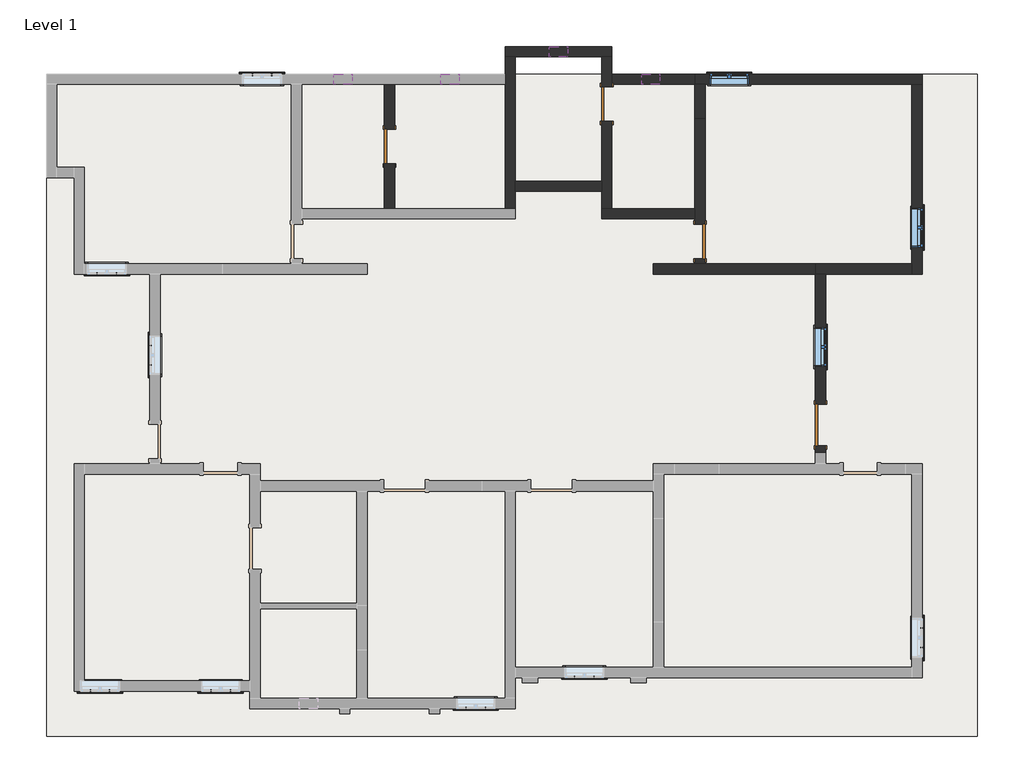
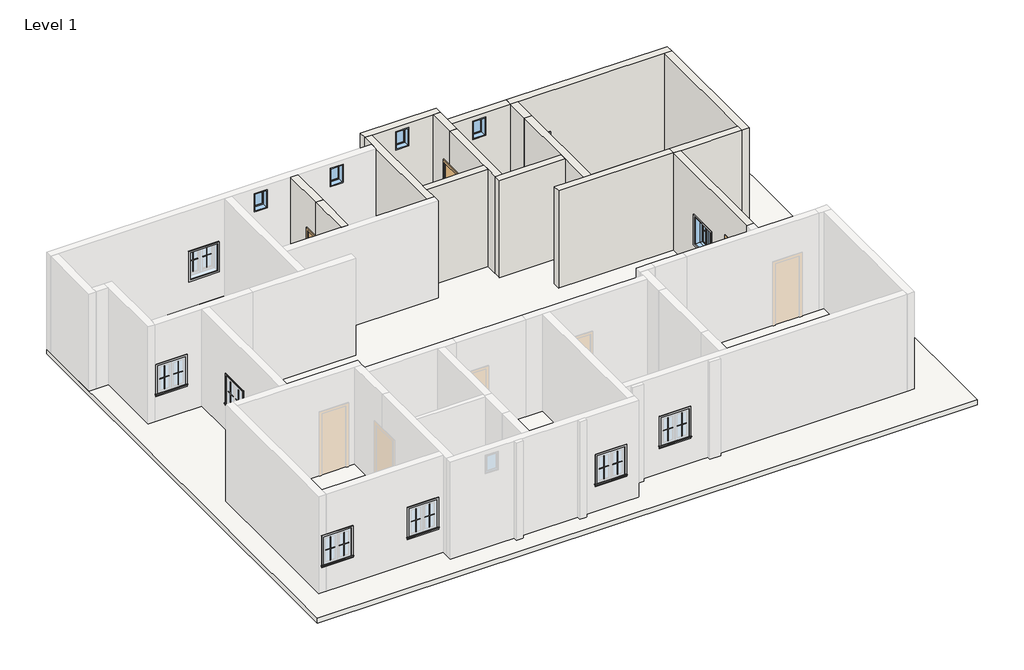
# One storey, part 2 of 2: 44 proxies, 16 walls, 7 windows, 4 doors, 1 slab.
"""IFC4 building model written with IfcOpenShell, lengths in millimetres."""

from ifc_helpers import new_model, si_unit, frame, origin, origin_with_axes, place, context, project, spatial, polyline, outline, extrude, faceted_brep, transform, mapped, element, save
from components import muntin_pattern_2x2_muntin_pattern_2x2_b3fe6957, muntin_pattern_2x2_muntin_pattern_2x2_3e0ecaf2, trim_window_exterior_flat_with_sill_41619996, trim_window_exterior_flat_with_sill_f2223f96, trim_window_interior_flat_picture_frame_51c85655, trim_window_interior_flat_picture_frame_1c9020d0, door_a1484949, door_a90ba1ad, window_aa618e30, window_339605e1, window_791baf9d

model = new_model("IFC4")

# Units and contexts
model_context = context("Model", 3, world=origin())
ifc_project = project(units=[si_unit("LENGTHUNIT", "METRE", prefix="MILLI")], contexts=[model_context])

# Site, building, storey
site = spatial("IfcSite", under=ifc_project)
building = spatial("IfcBuilding", under=site)
storey = spatial("IfcBuildingStorey", under=building, Name="Level 1", Elevation=0.0)

# Proxies
placement = place(None, origin())
muntin_pattern_2x2_muntin_pattern_2x2_shape = muntin_pattern_2x2_muntin_pattern_2x2_b3fe6957(model_context)
element("IfcBuildingElementProxy", 1, Name="Muntin Pattern_2x2 : Muntin Pattern_2x2", ObjectType="Muntin Pattern_2x2 : Muntin Pattern_2x2", at=placement, inside=storey, context=model_context, shape_type="MappedRepresentation", body=[
    mapped(muntin_pattern_2x2_muntin_pattern_2x2_shape, transform((-11799.4165084, 1543.0810985, 984.25), x_axis=(0.0, 1.0, 0.0), y_axis=(-1.0, 0.0, 0.0), z_axis=(0.0, 0.0, 1.0))),
])
element("IfcBuildingElementProxy", 2, Name="Muntin Pattern_2x2 : Muntin Pattern_2x2", ObjectType="Muntin Pattern_2x2 : Muntin Pattern_2x2", at=placement, inside=storey, context=model_context, shape_type="MappedRepresentation", body=[
    mapped(muntin_pattern_2x2_muntin_pattern_2x2_shape, transform((-12547.1290084, 3557.6185985, 984.25), x_axis=(-1.0, 0.0, 0.0), y_axis=(0.0, -1.0, 0.0), z_axis=(0.0, 0.0, 1.0))),
])
element("IfcBuildingElementProxy", 3, Name="Muntin Pattern_2x2 : Muntin Pattern_2x2", ObjectType="Muntin Pattern_2x2 : Muntin Pattern_2x2", at=placement, inside=storey, context=model_context, shape_type="MappedRepresentation", body=[
    mapped(muntin_pattern_2x2_muntin_pattern_2x2_shape, transform((5250.3334916, 4791.1060985, 984.25), x_axis=(0.0, -1.0, 0.0), y_axis=(1.0, 0.0, 0.0), z_axis=(0.0, 0.0, 1.0))),
])
element("IfcBuildingElementProxy", 4, Name="Muntin Pattern_2x2 : Muntin Pattern_2x2", ObjectType="Muntin Pattern_2x2 : Muntin Pattern_2x2", at=placement, inside=storey, context=model_context, shape_type="MappedRepresentation", body=[
    mapped(muntin_pattern_2x2_muntin_pattern_2x2_shape, transform((778.3459916, 7958.1685985, 984.25), x_axis=(1.0, 0.0, 0.0), y_axis=(0.0, 1.0, 0.0), z_axis=(0.0, 0.0, 1.0))),
])
element("IfcBuildingElementProxy", 5, Name="Muntin Pattern_2x2 : Muntin Pattern_2x2", ObjectType="Muntin Pattern_2x2 : Muntin Pattern_2x2", at=placement, inside=storey, context=model_context, shape_type="MappedRepresentation", body=[
    mapped(muntin_pattern_2x2_muntin_pattern_2x2_shape, transform((-9546.7540084, 7958.1685985, 984.25), x_axis=(1.0, 0.0, 0.0), y_axis=(0.0, 1.0, 0.0), z_axis=(0.0, 0.0, 1.0))),
])
element("IfcBuildingElementProxy", 6, Name="Muntin Pattern_2x2 : Muntin Pattern_2x2", ObjectType="Muntin Pattern_2x2 : Muntin Pattern_2x2", at=placement, inside=storey, context=model_context, shape_type="MappedRepresentation", body=[
    mapped(muntin_pattern_2x2_muntin_pattern_2x2_shape, transform((-12699.5290084, -5662.5814015, 984.25), x_axis=(-1.0, 0.0, 0.0), y_axis=(0.0, -1.0, 0.0), z_axis=(0.0, 0.0, 1.0))),
])
element("IfcBuildingElementProxy", 7, Name="Muntin Pattern_2x2 : Muntin Pattern_2x2", ObjectType="Muntin Pattern_2x2 : Muntin Pattern_2x2", at=placement, inside=storey, context=model_context, shape_type="MappedRepresentation", body=[
    mapped(muntin_pattern_2x2_muntin_pattern_2x2_shape, transform((-10032.5290084, -5662.5814015, 984.25), x_axis=(-1.0, 0.0, 0.0), y_axis=(0.0, -1.0, 0.0), z_axis=(0.0, 0.0, 1.0))),
])
element("IfcBuildingElementProxy", 8, Name="Muntin Pattern_2x2 : Muntin Pattern_2x2", ObjectType="Muntin Pattern_2x2 : Muntin Pattern_2x2", at=placement, inside=storey, context=model_context, shape_type="MappedRepresentation", body=[
    mapped(muntin_pattern_2x2_muntin_pattern_2x2_shape, transform((-4393.7290084, -6043.6598078, 984.25), x_axis=(-1.0, 0.0, 0.0), y_axis=(0.0, -1.0, 0.0), z_axis=(0.0, 0.0, 1.0))),
])
element("IfcBuildingElementProxy", 9, Name="Muntin Pattern_2x2 : Muntin Pattern_2x2", ObjectType="Muntin Pattern_2x2 : Muntin Pattern_2x2", at=placement, inside=storey, context=model_context, shape_type="MappedRepresentation", body=[
    mapped(muntin_pattern_2x2_muntin_pattern_2x2_shape, transform((5250.3334916, -4276.6939015, 984.25), x_axis=(0.0, -1.0, 0.0), y_axis=(1.0, 0.0, 0.0), z_axis=(0.0, 0.0, 1.0))),
])
element("IfcBuildingElementProxy", 10, Name="Muntin Pattern_2x2 : Muntin Pattern_2x2", ObjectType="Muntin Pattern_2x2 : Muntin Pattern_2x2", at=placement, inside=storey, context=model_context, shape_type="MappedRepresentation", body=[
    mapped(muntin_pattern_2x2_muntin_pattern_2x2_shape, transform((-1993.4290084, -5357.7814015, 984.25), x_axis=(-1.0, 0.0, 0.0), y_axis=(0.0, -1.0, 0.0), z_axis=(0.0, 0.0, 1.0))),
])
element("IfcBuildingElementProxy", 11, Name="Muntin Pattern_2x2 : Muntin Pattern_2x2", ObjectType="Muntin Pattern_2x2 : Muntin Pattern_2x2", at=placement, inside=storey, context=model_context, shape_type="MappedRepresentation", body=[
    mapped(muntin_pattern_2x2_muntin_pattern_2x2_shape, transform((3116.7334916, 2151.8097262, 984.25), x_axis=(0.0, -1.0, 0.0), y_axis=(1.0, 0.0, 0.0), z_axis=(0.0, 0.0, 1.0))),
])
muntin_pattern_2x2_muntin_pattern_2x2_2_shape = muntin_pattern_2x2_muntin_pattern_2x2_3e0ecaf2(model_context)
element("IfcBuildingElementProxy", 12, Name="Muntin Pattern_2x2 : Muntin Pattern_2x2", ObjectType="Muntin Pattern_2x2 : Muntin Pattern_2x2", at=placement, inside=storey, context=model_context, shape_type="MappedRepresentation", body=[
    mapped(muntin_pattern_2x2_muntin_pattern_2x2_2_shape, transform((-11799.4165084, 1971.7060985, 984.25), x_axis=(0.0, -1.0, 0.0), y_axis=(1.0, 0.0, 0.0), z_axis=(0.0, 0.0, 1.0))),
])
element("IfcBuildingElementProxy", 13, Name="Muntin Pattern_2x2 : Muntin Pattern_2x2", ObjectType="Muntin Pattern_2x2 : Muntin Pattern_2x2", at=placement, inside=storey, context=model_context, shape_type="MappedRepresentation", body=[
    mapped(muntin_pattern_2x2_muntin_pattern_2x2_2_shape, transform((-12975.7540084, 3557.6185985, 984.25), x_axis=(1.0, 0.0, 0.0), y_axis=(0.0, 1.0, 0.0), z_axis=(0.0, 0.0, 1.0))),
])
element("IfcBuildingElementProxy", 14, Name="Muntin Pattern_2x2 : Muntin Pattern_2x2", ObjectType="Muntin Pattern_2x2 : Muntin Pattern_2x2", at=placement, inside=storey, context=model_context, shape_type="MappedRepresentation", body=[
    mapped(muntin_pattern_2x2_muntin_pattern_2x2_2_shape, transform((5250.3334916, 4362.4810985, 984.25), x_axis=(0.0, 1.0, 0.0), y_axis=(-1.0, 0.0, 0.0), z_axis=(0.0, 0.0, 1.0))),
])
element("IfcBuildingElementProxy", 15, Name="Muntin Pattern_2x2 : Muntin Pattern_2x2", ObjectType="Muntin Pattern_2x2 : Muntin Pattern_2x2", at=placement, inside=storey, context=model_context, shape_type="MappedRepresentation", body=[
    mapped(muntin_pattern_2x2_muntin_pattern_2x2_2_shape, transform((1206.9709916, 7958.1685985, 984.25), x_axis=(-1.0, 0.0, 0.0), y_axis=(0.0, -1.0, 0.0), z_axis=(0.0, 0.0, 1.0))),
])
element("IfcBuildingElementProxy", 16, Name="Muntin Pattern_2x2 : Muntin Pattern_2x2", ObjectType="Muntin Pattern_2x2 : Muntin Pattern_2x2", at=placement, inside=storey, context=model_context, shape_type="MappedRepresentation", body=[
    mapped(muntin_pattern_2x2_muntin_pattern_2x2_2_shape, transform((-9118.1290084, 7958.1685985, 984.25), x_axis=(-1.0, 0.0, 0.0), y_axis=(0.0, -1.0, 0.0), z_axis=(0.0, 0.0, 1.0))),
])
element("IfcBuildingElementProxy", 17, Name="Muntin Pattern_2x2 : Muntin Pattern_2x2", ObjectType="Muntin Pattern_2x2 : Muntin Pattern_2x2", at=placement, inside=storey, context=model_context, shape_type="MappedRepresentation", body=[
    mapped(muntin_pattern_2x2_muntin_pattern_2x2_2_shape, transform((-13128.1540084, -5662.5814015, 984.25), x_axis=(1.0, 0.0, 0.0), y_axis=(0.0, 1.0, 0.0), z_axis=(0.0, 0.0, 1.0))),
])
element("IfcBuildingElementProxy", 18, Name="Muntin Pattern_2x2 : Muntin Pattern_2x2", ObjectType="Muntin Pattern_2x2 : Muntin Pattern_2x2", at=placement, inside=storey, context=model_context, shape_type="MappedRepresentation", body=[
    mapped(muntin_pattern_2x2_muntin_pattern_2x2_2_shape, transform((-10461.1540084, -5662.5814015, 984.25), x_axis=(1.0, 0.0, 0.0), y_axis=(0.0, 1.0, 0.0), z_axis=(0.0, 0.0, 1.0))),
])
element("IfcBuildingElementProxy", 19, Name="Muntin Pattern_2x2 : Muntin Pattern_2x2", ObjectType="Muntin Pattern_2x2 : Muntin Pattern_2x2", at=placement, inside=storey, context=model_context, shape_type="MappedRepresentation", body=[
    mapped(muntin_pattern_2x2_muntin_pattern_2x2_2_shape, transform((-4822.3540084, -6043.6598078, 984.25), x_axis=(1.0, 0.0, 0.0), y_axis=(0.0, 1.0, 0.0), z_axis=(0.0, 0.0, 1.0))),
])
element("IfcBuildingElementProxy", 20, Name="Muntin Pattern_2x2 : Muntin Pattern_2x2", ObjectType="Muntin Pattern_2x2 : Muntin Pattern_2x2", at=placement, inside=storey, context=model_context, shape_type="MappedRepresentation", body=[
    mapped(muntin_pattern_2x2_muntin_pattern_2x2_2_shape, transform((5250.3334916, -4705.3189015, 984.25), x_axis=(0.0, 1.0, 0.0), y_axis=(-1.0, 0.0, 0.0), z_axis=(0.0, 0.0, 1.0))),
])
element("IfcBuildingElementProxy", 21, Name="Muntin Pattern_2x2 : Muntin Pattern_2x2", ObjectType="Muntin Pattern_2x2 : Muntin Pattern_2x2", at=placement, inside=storey, context=model_context, shape_type="MappedRepresentation", body=[
    mapped(muntin_pattern_2x2_muntin_pattern_2x2_2_shape, transform((-2422.0540084, -5357.7814015, 984.25), x_axis=(1.0, 0.0, 0.0), y_axis=(0.0, 1.0, 0.0), z_axis=(0.0, 0.0, 1.0))),
])
element("IfcBuildingElementProxy", 22, Name="Muntin Pattern_2x2 : Muntin Pattern_2x2", ObjectType="Muntin Pattern_2x2 : Muntin Pattern_2x2", at=placement, inside=storey, context=model_context, shape_type="MappedRepresentation", body=[
    mapped(muntin_pattern_2x2_muntin_pattern_2x2_2_shape, transform((3116.7334916, 1723.1847262, 984.25), x_axis=(0.0, 1.0, 0.0), y_axis=(-1.0, 0.0, 0.0), z_axis=(0.0, 0.0, 1.0))),
])
trim_window_exterior_flat_with_sill_shape = trim_window_exterior_flat_with_sill_41619996(model_context)
element("IfcBuildingElementProxy", 23, Name="Trim-Window-Exterior-Flat : with Sill", ObjectType="Trim-Window-Exterior-Flat : with Sill", at=placement, inside=storey, context=model_context, shape_type="MappedRepresentation", body=[
    mapped(trim_window_exterior_flat_with_sill_shape, transform((-11808.9415084, 1757.3935985, 1828.8), x_axis=(0.0, -1.0, 0.0), y_axis=(0.0, 0.0, 1.0), z_axis=(-1.0, 0.0, 0.0))),
])
element("IfcBuildingElementProxy", 24, Name="Trim-Window-Exterior-Flat : with Sill", ObjectType="Trim-Window-Exterior-Flat : with Sill", at=placement, inside=storey, context=model_context, shape_type="MappedRepresentation", body=[
    mapped(trim_window_exterior_flat_with_sill_shape, transform((-12761.4415084, 3548.0935985, 1828.8), x_axis=(1.0, 0.0, 0.0), y_axis=(0.0, 0.0, 1.0), z_axis=(0.0, -1.0, 0.0))),
])
element("IfcBuildingElementProxy", 25, Name="Trim-Window-Exterior-Flat : with Sill", ObjectType="Trim-Window-Exterior-Flat : with Sill", at=placement, inside=storey, context=model_context, shape_type="MappedRepresentation", body=[
    mapped(trim_window_exterior_flat_with_sill_shape, transform((5259.8584916, 4576.7935985, 1828.8), x_axis=(0.0, 1.0, 0.0), y_axis=(0.0, 0.0, 1.0), z_axis=(1.0, 0.0, 0.0))),
])
element("IfcBuildingElementProxy", 26, Name="Trim-Window-Exterior-Flat : with Sill", ObjectType="Trim-Window-Exterior-Flat : with Sill", at=placement, inside=storey, context=model_context, shape_type="MappedRepresentation", body=[
    mapped(trim_window_exterior_flat_with_sill_shape, transform((992.6584916, 7967.6935985, 1828.8), x_axis=(-1.0, 0.0, 0.0), y_axis=(0.0, 0.0, 1.0), z_axis=(0.0, 1.0, 0.0))),
])
element("IfcBuildingElementProxy", 27, Name="Trim-Window-Exterior-Flat : with Sill", ObjectType="Trim-Window-Exterior-Flat : with Sill", at=placement, inside=storey, context=model_context, shape_type="MappedRepresentation", body=[
    mapped(trim_window_exterior_flat_with_sill_shape, transform((-9332.4415084, 7967.6935985, 1828.8), x_axis=(-1.0, 0.0, 0.0), y_axis=(0.0, 0.0, 1.0), z_axis=(0.0, 1.0, 0.0))),
])
element("IfcBuildingElementProxy", 28, Name="Trim-Window-Exterior-Flat : with Sill", ObjectType="Trim-Window-Exterior-Flat : with Sill", at=placement, inside=storey, context=model_context, shape_type="MappedRepresentation", body=[
    mapped(trim_window_exterior_flat_with_sill_shape, transform((-12913.8415084, -5672.1064015, 1828.8), x_axis=(1.0, 0.0, 0.0), y_axis=(0.0, 0.0, 1.0), z_axis=(0.0, -1.0, 0.0))),
])
element("IfcBuildingElementProxy", 29, Name="Trim-Window-Exterior-Flat : with Sill", ObjectType="Trim-Window-Exterior-Flat : with Sill", at=placement, inside=storey, context=model_context, shape_type="MappedRepresentation", body=[
    mapped(trim_window_exterior_flat_with_sill_shape, transform((-10246.8415084, -5672.1064015, 1828.8), x_axis=(1.0, 0.0, 0.0), y_axis=(0.0, 0.0, 1.0), z_axis=(0.0, -1.0, 0.0))),
])
element("IfcBuildingElementProxy", 30, Name="Trim-Window-Exterior-Flat : with Sill", ObjectType="Trim-Window-Exterior-Flat : with Sill", at=placement, inside=storey, context=model_context, shape_type="MappedRepresentation", body=[
    mapped(trim_window_exterior_flat_with_sill_shape, transform((-4608.0415084, -6053.1848078, 1828.8), x_axis=(1.0, 0.0, 0.0), y_axis=(0.0, 0.0, 1.0), z_axis=(0.0, -1.0, 0.0))),
])
element("IfcBuildingElementProxy", 31, Name="Trim-Window-Exterior-Flat : with Sill", ObjectType="Trim-Window-Exterior-Flat : with Sill", at=placement, inside=storey, context=model_context, shape_type="MappedRepresentation", body=[
    mapped(trim_window_exterior_flat_with_sill_shape, transform((5259.8584916, -4491.0064015, 1828.8), x_axis=(0.0, 1.0, 0.0), y_axis=(0.0, 0.0, 1.0), z_axis=(1.0, 0.0, 0.0))),
])
trim_window_exterior_flat_with_sill_2_shape = trim_window_exterior_flat_with_sill_f2223f96(model_context)
element("IfcBuildingElementProxy", 32, Name="Trim-Window-Exterior-Flat : with Sill", ObjectType="Trim-Window-Exterior-Flat : with Sill", at=placement, inside=storey, context=model_context, shape_type="MappedRepresentation", body=[
    mapped(trim_window_exterior_flat_with_sill_2_shape, transform((-2207.7415084, -5367.3064015, 1828.8), x_axis=(-1.0, 0.0, 0.0), y_axis=(0.0, 0.0, -1.0), z_axis=(0.0, -1.0, 0.0))),
])
element("IfcBuildingElementProxy", 33, Name="Trim-Window-Exterior-Flat : with Sill", ObjectType="Trim-Window-Exterior-Flat : with Sill", at=placement, inside=storey, context=model_context, shape_type="MappedRepresentation", body=[
    mapped(trim_window_exterior_flat_with_sill_2_shape, transform((3126.2584916, 1937.4972262, 1828.8), x_axis=(0.0, -1.0, 0.0), y_axis=(0.0, 0.0, -1.0), z_axis=(1.0, 0.0, 0.0))),
])
trim_window_interior_flat_picture_frame_shape = trim_window_interior_flat_picture_frame_51c85655(model_context)
element("IfcBuildingElementProxy", 34, Name="Trim-Window-Interior-Flat : Picture Frame", ObjectType="Trim-Window-Interior-Flat : Picture Frame", at=placement, inside=storey, context=model_context, shape_type="MappedRepresentation", body=[
    mapped(trim_window_interior_flat_picture_frame_shape, transform((-11580.3415084, 1757.3935985, 1828.8), x_axis=(0.0, 1.0, 0.0), y_axis=(0.0, 0.0, 1.0), z_axis=(1.0, 0.0, 0.0))),
])
element("IfcBuildingElementProxy", 35, Name="Trim-Window-Interior-Flat : Picture Frame", ObjectType="Trim-Window-Interior-Flat : Picture Frame", at=placement, inside=storey, context=model_context, shape_type="MappedRepresentation", body=[
    mapped(trim_window_interior_flat_picture_frame_shape, transform((-12761.4415084, 3776.6935985, 1828.8), x_axis=(-1.0, 0.0, 0.0), y_axis=(0.0, 0.0, 1.0), z_axis=(0.0, 1.0, 0.0))),
])
element("IfcBuildingElementProxy", 36, Name="Trim-Window-Interior-Flat : Picture Frame", ObjectType="Trim-Window-Interior-Flat : Picture Frame", at=placement, inside=storey, context=model_context, shape_type="MappedRepresentation", body=[
    mapped(trim_window_interior_flat_picture_frame_shape, transform((5031.2584916, 4576.7935985, 1828.8), x_axis=(0.0, -1.0, 0.0), y_axis=(0.0, 0.0, 1.0), z_axis=(-1.0, 0.0, 0.0))),
])
element("IfcBuildingElementProxy", 37, Name="Trim-Window-Interior-Flat : Picture Frame", ObjectType="Trim-Window-Interior-Flat : Picture Frame", at=placement, inside=storey, context=model_context, shape_type="MappedRepresentation", body=[
    mapped(trim_window_interior_flat_picture_frame_shape, transform((992.6584916, 7739.0935985, 1828.8), x_axis=(1.0, 0.0, 0.0), y_axis=(0.0, 0.0, 1.0), z_axis=(0.0, -1.0, 0.0))),
])
element("IfcBuildingElementProxy", 38, Name="Trim-Window-Interior-Flat : Picture Frame", ObjectType="Trim-Window-Interior-Flat : Picture Frame", at=placement, inside=storey, context=model_context, shape_type="MappedRepresentation", body=[
    mapped(trim_window_interior_flat_picture_frame_shape, transform((-9332.4415084, 7739.0935985, 1828.8), x_axis=(1.0, 0.0, 0.0), y_axis=(0.0, 0.0, 1.0), z_axis=(0.0, -1.0, 0.0))),
])
element("IfcBuildingElementProxy", 39, Name="Trim-Window-Interior-Flat : Picture Frame", ObjectType="Trim-Window-Interior-Flat : Picture Frame", at=placement, inside=storey, context=model_context, shape_type="MappedRepresentation", body=[
    mapped(trim_window_interior_flat_picture_frame_shape, transform((-12913.8415084, -5443.5064015, 1828.8), x_axis=(-1.0, 0.0, 0.0), y_axis=(0.0, 0.0, 1.0), z_axis=(0.0, 1.0, 0.0))),
])
element("IfcBuildingElementProxy", 40, Name="Trim-Window-Interior-Flat : Picture Frame", ObjectType="Trim-Window-Interior-Flat : Picture Frame", at=placement, inside=storey, context=model_context, shape_type="MappedRepresentation", body=[
    mapped(trim_window_interior_flat_picture_frame_shape, transform((-10246.8415084, -5443.5064015, 1828.8), x_axis=(-1.0, 0.0, 0.0), y_axis=(0.0, 0.0, 1.0), z_axis=(0.0, 1.0, 0.0))),
])
element("IfcBuildingElementProxy", 41, Name="Trim-Window-Interior-Flat : Picture Frame", ObjectType="Trim-Window-Interior-Flat : Picture Frame", at=placement, inside=storey, context=model_context, shape_type="MappedRepresentation", body=[
    mapped(trim_window_interior_flat_picture_frame_shape, transform((-4608.0415084, -5824.5848078, 1828.8), x_axis=(-1.0, 0.0, 0.0), y_axis=(0.0, 0.0, 1.0), z_axis=(0.0, 1.0, 0.0))),
])
element("IfcBuildingElementProxy", 42, Name="Trim-Window-Interior-Flat : Picture Frame", ObjectType="Trim-Window-Interior-Flat : Picture Frame", at=placement, inside=storey, context=model_context, shape_type="MappedRepresentation", body=[
    mapped(trim_window_interior_flat_picture_frame_shape, transform((5031.2584916, -4491.0064015, 1828.8), x_axis=(0.0, -1.0, 0.0), y_axis=(0.0, 0.0, 1.0), z_axis=(-1.0, 0.0, 0.0))),
])
trim_window_interior_flat_picture_frame_2_shape = trim_window_interior_flat_picture_frame_1c9020d0(model_context)
element("IfcBuildingElementProxy", 43, Name="Trim-Window-Interior-Flat : Picture Frame", ObjectType="Trim-Window-Interior-Flat : Picture Frame", at=placement, inside=storey, context=model_context, shape_type="MappedRepresentation", body=[
    mapped(trim_window_interior_flat_picture_frame_2_shape, transform((-2207.7415084, -5138.7064015, 1828.8), x_axis=(1.0, 0.0, 0.0), y_axis=(0.0, 0.0, -1.0), z_axis=(0.0, 1.0, 0.0))),
])
element("IfcBuildingElementProxy", 44, Name="Trim-Window-Interior-Flat : Picture Frame", ObjectType="Trim-Window-Interior-Flat : Picture Frame", at=placement, inside=storey, context=model_context, shape_type="MappedRepresentation", body=[
    mapped(trim_window_interior_flat_picture_frame_2_shape, transform((2897.6584916, 1937.4972262, 1828.8), x_axis=(0.0, 1.0, 0.0), y_axis=(0.0, 0.0, -1.0), z_axis=(-1.0, 0.0, 0.0))),
])

# Doors
door_shape = door_a1484949(model_context)
element("IfcDoor", 45, ObjectType="Single-Flush : 30\" x 80\"", at=placement, inside=storey, context=model_context, shape_type="MappedRepresentation", body=[
    mapped(door_shape, transform((344.9584916, 4271.9935985, 0.0), x_axis=(0.0, -1.0, 0.0), y_axis=(1.0, 0.0, 0.0), z_axis=(0.0, 0.0, 1.0))),
])
element("IfcDoor", 46, ObjectType="Single-Flush : 30\" x 80\"", at=placement, inside=storey, context=model_context, shape_type="MappedRepresentation", body=[
    mapped(door_shape, transform((-6513.0415084, 6367.4935985, 0.0), x_axis=(0.0, 1.0, 0.0), y_axis=(-1.0, 0.0, 0.0), z_axis=(0.0, 0.0, 1.0))),
])
element("IfcDoor", 47, ObjectType="Single-Flush : 30\" x 80\"", at=placement, inside=storey, context=model_context, shape_type="MappedRepresentation", body=[
    mapped(door_shape, transform((-1712.4415084, 7305.508295, 0.0), x_axis=(0.0, 1.0, 0.0), y_axis=(-1.0, 0.0, 0.0), z_axis=(0.0, 0.0, 1.0))),
])
door_2_shape = door_a90ba1ad(model_context)
element("IfcDoor", 48, ObjectType="Single-Flush : 36\" x 84\"", at=placement, inside=storey, context=model_context, shape_type="MappedRepresentation", body=[
    mapped(door_2_shape, transform((3011.9584916, 212.600854, 0.0), x_axis=(0.0, -1.0, 0.0), y_axis=(1.0, 0.0, 0.0), z_axis=(0.0, 0.0, 1.0))),
])

# Slab
element("IfcSlab", 49, ObjectType="6\"", at=placement, inside=storey, context=model_context, shape_type="SweptSolid", body=[
    extrude(outline(polyline([(6479.0584916, 7967.6935985), (6479.0584916, -6662.7064015), (-14094.9415084, -6662.7064015), (-14094.9415084, 7967.6935985), (6479.0584916, 7967.6935985)])), frame((0.0, 0.0, -152.4), z_axis=(0.0, 0.0, 1.0), x_axis=(1.0, 0.0, 0.0)), (0.0, 0.0, 1.0), 152.4),
])

# Walls
element("IfcWall", 50, ObjectType="9\"", at=placement, inside=storey, context=model_context, shape_type="Brep", body=[
    faceted_brep([(-1598.1415084, 8577.2935985, 0.0), (-3960.3415084, 8577.2935985, 0.0), (-3960.3415084, 8577.2935985, 3200.4), (-1598.1415084, 8577.2935985, 3200.4), (-2576.0415084, 8577.2935985, 3048.0), (-2982.4415084, 8577.2935985, 3048.0), (-2982.4415084, 8577.2935985, 2438.4), (-2576.0415084, 8577.2935985, 2438.4), (-1598.1415084, 8348.6935985, 0.0), (-1598.1415084, 8348.6935985, 3200.4), (-1826.7415084, 8348.6935985, 3200.4), (-3731.7415084, 8348.6935985, 3200.4), (-3960.3415084, 8348.6935985, 3200.4), (-3960.3415084, 8348.6935985, 0.0), (-3731.7415084, 8348.6935985, 0.0), (-1826.7415084, 8348.6935985, 0.0), (-2576.0415084, 8348.6935985, 3048.0), (-2576.0415084, 8348.6935985, 2438.4), (-2982.4415084, 8348.6935985, 2438.4), (-2982.4415084, 8348.6935985, 3048.0)], [[[0, 1, 2, 3], [4, 5, 6, 7]], [[8, 9, 10, 11, 12, 13, 14, 15], [16, 17, 18, 19]], [[1, 0, 8, 15, 14, 13]], [[3, 2, 12, 11, 10, 9]], [[2, 1, 13, 12]], [[0, 3, 9, 8]], [[17, 16, 4, 7]], [[18, 17, 7, 6]], [[19, 18, 6, 5]], [[16, 19, 5, 4]]]),
])
element("IfcWall", 51, ObjectType="9\"", at=placement, inside=storey, context=model_context, shape_type="Brep", body=[
    faceted_brep([(5259.8584916, 7967.6935985, 0.0), (230.6584916, 7967.6935985, 0.0), (230.6584916, 7967.6935985, 3200.4), (5259.8584916, 7967.6935985, 3200.4), (1424.4584916, 7967.6935985, 1828.8), (560.8584916, 7967.6935985, 1828.8), (560.8584916, 7967.6935985, 914.4), (1424.4584916, 7967.6935985, 914.4), (5259.8584916, 7739.0935985, 0.0), (5259.8584916, 7739.0935985, 3200.4), (5031.2584916, 7739.0935985, 3200.4), (459.2584916, 7739.0935985, 3200.4), (230.6584916, 7739.0935985, 3200.4), (230.6584916, 7739.0935985, 0.0), (459.2584916, 7739.0935985, 0.0), (5031.2584916, 7739.0935985, 0.0), (1424.4584916, 7739.0935985, 1828.8), (1424.4584916, 7739.0935985, 914.4), (560.8584916, 7739.0935985, 914.4), (560.8584916, 7739.0935985, 1828.8)], [[[0, 1, 2, 3], [4, 5, 6, 7]], [[8, 9, 10, 11, 12, 13, 14, 15], [16, 17, 18, 19]], [[1, 0, 8, 15, 14, 13]], [[3, 2, 12, 11, 10, 9]], [[2, 1, 13, 12]], [[0, 3, 9, 8]], [[17, 16, 4, 7]], [[18, 17, 7, 6]], [[19, 18, 6, 5]], [[16, 19, 5, 4]]]),
])
element("IfcWall", 52, ObjectType="9\"", at=placement, inside=storey, context=model_context, shape_type="SweptSolid", body=[
    extrude(outline(polyline([(0.0, 230.6584916), (3200.4, 230.6584916), (3200.4, -1598.1415084), (0.0, -1598.1415084), (0.0, 230.6584916)]), holes=[polyline([(3048.0, -537.6915084), (2438.4, -537.6915084), (2438.4, -944.0915084), (3048.0, -944.0915084), (3048.0, -537.6915084)])]), frame((0.0, 7739.0935985, 0.0), z_axis=(0.0, 1.0, 0.0), x_axis=(0.0, 0.0, 1.0)), (0.0, 0.0, 1.0), 228.6),
])
element("IfcWall", 53, ObjectType="9\"", at=placement, inside=storey, context=model_context, shape_type="SweptSolid", body=[
    extrude(outline(polyline([(230.6584916, 6983.3288801), (230.6584916, 7739.0935985), (459.2584916, 7739.0935985), (459.2584916, 6983.3288801), (230.6584916, 6983.3288801)])), origin_with_axes(), (0.0, 0.0, 1.0), 3200.4),
])
element("IfcWall", 54, ObjectType="9\"", at=placement, inside=storey, context=model_context, shape_type="Brep", body=[
    faceted_brep([(230.6584916, 4995.8935985, 0.0), (-1598.1415084, 4995.8935985, 0.0), (-1826.7415084, 4995.8935985, 0.0), (-1826.7415084, 4995.8935985, 3200.4), (-1598.1415084, 4995.8935985, 3200.4), (230.6584916, 4995.8935985, 3200.4), (230.6584916, 4767.2935985, 0.0), (230.6584916, 4767.2935985, 3200.4), (-1826.7415084, 4767.2935985, 3200.4), (-1826.7415084, 4767.2935985, 0.0)], [[[0, 1, 2, 3, 4, 5]], [[6, 7, 8, 9]], [[2, 1, 0, 6, 9]], [[5, 4, 3, 8, 7]], [[0, 5, 7, 6]], [[3, 2, 9, 8]]]),
])
element("IfcWall", 55, ObjectType="9\"", at=placement, inside=storey, context=model_context, shape_type="SweptSolid", body=[
    extrude(outline(polyline([(6367.4935985, 3200.4), (7739.0935985, 3200.4), (7739.0935985, 0.0), (6748.4935985, 0.0), (6748.4935985, 2032.0), (6367.4935985, 2032.0), (6367.4935985, 3200.4)])), frame((-6627.3415084, 0.0, 0.0), z_axis=(1.0, 0.0, 0.0), x_axis=(0.0, 1.0, 0.0)), (0.0, 0.0, 1.0), 228.6),
])
element("IfcWall", 56, ObjectType="9\"", at=placement, inside=storey, context=model_context, shape_type="SweptSolid", body=[
    extrude(outline(polyline([(4995.8935985, 3200.4), (6367.4935985, 3200.4), (6367.4935985, 2032.0), (5986.4935985, 2032.0), (5986.4935985, 0.0), (4995.8935985, 0.0), (4995.8935985, 3200.4)])), frame((-6627.3415084, 0.0, 0.0), z_axis=(1.0, 0.0, 0.0), x_axis=(0.0, 1.0, 0.0)), (0.0, 0.0, 1.0), 228.6),
])
element("IfcWall", 57, ObjectType="9\"", at=placement, inside=storey, context=model_context, shape_type="Brep", body=[
    faceted_brep([(-3960.3415084, 8348.6935985, 0.0), (-3960.3415084, 7967.6935985, 0.0), (-3960.3415084, 7739.0935985, 0.0), (-3960.3415084, 4995.8935985, 0.0), (-3960.3415084, 4995.8935985, 3200.4), (-3960.3415084, 7739.0935985, 3200.4), (-3960.3415084, 7967.6935985, 3200.4), (-3960.3415084, 8348.6935985, 3200.4), (-3731.7415084, 8348.6935985, 0.0), (-3731.7415084, 8348.6935985, 3200.4), (-3731.7415084, 5605.4935985, 3200.4), (-3731.7415084, 5376.8935985, 3200.4), (-3731.7415084, 4995.8935985, 3200.4), (-3731.7415084, 4995.8935985, 0.0), (-3731.7415084, 5376.8935985, 0.0), (-3731.7415084, 5605.4935985, 0.0)], [[[0, 1, 2, 3, 4, 5, 6, 7]], [[8, 9, 10, 11, 12, 13, 14, 15]], [[3, 2, 1, 0, 8, 15, 14, 13]], [[7, 6, 5, 4, 12, 11, 10, 9]], [[0, 7, 9, 8]], [[4, 3, 13, 12]]]),
])
element("IfcWall", 58, ObjectType="9\"", at=placement, inside=storey, context=model_context, shape_type="Brep", body=[
    faceted_brep([(230.6584916, 3890.9935985, 2032.0), (230.6584916, 3890.9935985, 0.0), (230.6584916, 3776.6935985, 0.0), (230.6584916, 3776.6935985, 3200.4), (230.6584916, 4767.2935985, 3200.4), (230.6584916, 4995.8935985, 3200.4), (230.6584916, 6983.3288801, 3200.4), (230.6584916, 6983.3288801, 0.0), (230.6584916, 4995.8935985, 0.0), (230.6584916, 4767.2935985, 0.0), (230.6584916, 4652.9935985, 0.0), (230.6584916, 4652.9935985, 2032.0), (459.2584916, 3776.6935985, 0.0), (459.2584916, 3890.9935985, 0.0), (459.2584916, 3890.9935985, 2032.0), (459.2584916, 4652.9935985, 2032.0), (459.2584916, 4652.9935985, 0.0), (459.2584916, 6983.3288801, 0.0), (459.2584916, 6983.3288801, 3200.4), (459.2584916, 3776.6935985, 3200.4)], [[[0, 1, 2, 3, 4, 5, 6, 7, 8, 9, 10, 11]], [[12, 13, 14, 15, 16, 17, 18, 19]], [[2, 1, 13, 12]], [[10, 9, 8, 7, 17, 16]], [[6, 5, 4, 3, 19, 18]], [[7, 6, 18, 17]], [[3, 2, 12, 19]], [[14, 13, 1, 0]], [[15, 14, 0, 11]], [[16, 15, 11, 10]]]),
])
element("IfcWall", 59, ObjectType="9\"", at=placement, inside=storey, context=model_context, shape_type="Brep", body=[
    faceted_brep([(5031.2584916, 7739.0935985, 0.0), (5031.2584916, 3776.6935985, 0.0), (5031.2584916, 3548.0935985, 0.0), (5031.2584916, 3548.0935985, 3200.4), (5031.2584916, 3776.6935985, 3200.4), (5031.2584916, 7739.0935985, 3200.4), (5031.2584916, 4144.9935985, 1828.8), (5031.2584916, 4144.9935985, 914.4), (5031.2584916, 5008.5935985, 914.4), (5031.2584916, 5008.5935985, 1828.8), (5259.8584916, 7739.0935985, 0.0), (5259.8584916, 7739.0935985, 3200.4), (5259.8584916, 3548.0935985, 3200.4), (5259.8584916, 3548.0935985, 0.0), (5259.8584916, 4144.9935985, 1828.8), (5259.8584916, 5008.5935985, 1828.8), (5259.8584916, 5008.5935985, 914.4), (5259.8584916, 4144.9935985, 914.4)], [[[0, 1, 2, 3, 4, 5], [6, 7, 8, 9]], [[10, 11, 12, 13], [14, 15, 16, 17]], [[2, 1, 0, 10, 13]], [[5, 4, 3, 12, 11]], [[0, 5, 11, 10]], [[3, 2, 13, 12]], [[7, 6, 14, 17]], [[8, 7, 17, 16]], [[9, 8, 16, 15]], [[6, 9, 15, 14]]]),
])
element("IfcWall", 60, ObjectType="9\"", at=placement, inside=storey, context=model_context, shape_type="Brep", body=[
    faceted_brep([(5031.2584916, 3776.6935985, 0.0), (2897.6584916, 3776.6935985, 0.0), (2897.6584916, 3776.6935985, 3200.4), (5031.2584916, 3776.6935985, 3200.4), (5031.2584916, 3548.0935985, 0.0), (5031.2584916, 3548.0935985, 3200.4), (3126.2584916, 3548.0935985, 3200.4), (2897.6584916, 3548.0935985, 3200.4), (2897.6584916, 3548.0935985, 0.0), (3126.2584916, 3548.0935985, 0.0)], [[[0, 1, 2, 3]], [[4, 5, 6, 7, 8, 9]], [[1, 0, 4, 9, 8]], [[3, 2, 7, 6, 5]], [[0, 3, 5, 4]], [[2, 1, 8, 7]]]),
])
element("IfcWall", 61, ObjectType="9\"", at=placement, inside=storey, context=model_context, shape_type="SweptSolid", body=[
    extrude(outline(polyline([(-244.599146, 2133.6), (-244.599146, 0.0), (-396.999146, 0.0), (-396.999146, 3200.4), (3548.0935985, 3200.4), (3548.0935985, 0.0), (669.800854, 0.0), (669.800854, 2133.6), (-244.599146, 2133.6)]), holes=[polyline([(2369.2972262, 1828.8), (1505.6972262, 1828.8), (1505.6972262, 914.4), (2369.2972262, 914.4), (2369.2972262, 1828.8)])]), frame((2897.6584916, 0.0, 0.0), z_axis=(1.0, 0.0, 0.0), x_axis=(0.0, 1.0, 0.0)), (0.0, 0.0, 1.0), 228.6),
])
element("IfcWall", 62, ObjectType="9\"", at=placement, inside=storey, context=model_context, shape_type="Brep", body=[
    faceted_brep([(-1826.7415084, 4995.8935985, 3200.4), (-1826.7415084, 5376.8935985, 3200.4), (-1826.7415084, 5605.4935985, 3200.4), (-1826.7415084, 7457.908295, 3200.4), (-1826.7415084, 7457.908295, 2032.0), (-1826.7415084, 6924.508295, 2032.0), (-1826.7415084, 6924.508295, 0.0), (-1826.7415084, 5605.4935985, 0.0), (-1826.7415084, 5376.8935985, 0.0), (-1826.7415084, 4995.8935985, 0.0), (-1598.1415084, 7457.908295, 3200.4), (-1598.1415084, 4995.8935985, 3200.4), (-1598.1415084, 4995.8935985, 0.0), (-1598.1415084, 6924.508295, 0.0), (-1598.1415084, 6924.508295, 2032.0), (-1598.1415084, 7457.908295, 2032.0)], [[[0, 1, 2, 3, 4, 5, 6, 7, 8, 9]], [[10, 11, 12, 13, 14, 15]], [[12, 9, 8, 7, 6, 13]], [[3, 2, 1, 0, 11, 10]], [[3, 10, 15, 4]], [[0, 9, 12, 11]], [[14, 5, 4, 15]], [[5, 14, 13, 6]]]),
])
element("IfcWall", 63, ObjectType="9\"", at=placement, inside=storey, context=model_context, shape_type="SweptSolid", body=[
    extrude(outline(polyline([(-3731.7415084, 5605.4935985), (-1826.7415084, 5605.4935985), (-1826.7415084, 5376.8935985), (-3731.7415084, 5376.8935985), (-3731.7415084, 5605.4935985)])), origin_with_axes(), (0.0, 0.0, 1.0), 3200.4),
])
element("IfcWall", 64, ObjectType="9\"", at=placement, inside=storey, context=model_context, shape_type="Brep", body=[
    faceted_brep([(-1598.1415084, 8348.6935985, 3200.4), (-1598.1415084, 7967.6935985, 3200.4), (-1598.1415084, 7739.0935985, 3200.4), (-1598.1415084, 7457.908295, 3200.4), (-1598.1415084, 7457.908295, 2032.0), (-1598.1415084, 7686.508295, 2032.0), (-1598.1415084, 7686.508295, 0.0), (-1598.1415084, 7739.0935985, 0.0), (-1598.1415084, 7967.6935985, 0.0), (-1598.1415084, 8348.6935985, 0.0), (-1826.7415084, 7457.908295, 3200.4), (-1826.7415084, 8348.6935985, 3200.4), (-1826.7415084, 8348.6935985, 0.0), (-1826.7415084, 7686.508295, 0.0), (-1826.7415084, 7686.508295, 2032.0), (-1826.7415084, 7457.908295, 2032.0)], [[[0, 1, 2, 3, 4, 5, 6, 7, 8, 9]], [[10, 11, 12, 13, 14, 15]], [[12, 9, 8, 7, 6, 13]], [[3, 2, 1, 0, 11, 10]], [[3, 10, 15, 4]], [[0, 9, 12, 11]], [[14, 5, 4, 15]], [[5, 14, 13, 6]]]),
])
element("IfcWall", 65, ObjectType="9\"", at=placement, inside=storey, context=model_context, shape_type="Brep", body=[
    faceted_brep([(2897.6584916, 3776.6935985, 0.0), (459.2584916, 3776.6935985, 0.0), (230.6584916, 3776.6935985, 0.0), (-683.7415084, 3776.6935985, 0.0), (-683.7415084, 3776.6935985, 3200.4), (230.6584916, 3776.6935985, 3200.4), (459.2584916, 3776.6935985, 3200.4), (2897.6584916, 3776.6935985, 3200.4), (2897.6584916, 3548.0935985, 0.0), (2897.6584916, 3548.0935985, 3200.4), (-683.7415084, 3548.0935985, 3200.4), (-683.7415084, 3548.0935985, 0.0)], [[[0, 1, 2, 3, 4, 5, 6, 7]], [[8, 9, 10, 11]], [[3, 2, 1, 0, 8, 11]], [[4, 3, 11, 10]], [[7, 6, 5, 4, 10, 9]], [[0, 7, 9, 8]]]),
])

# Windows
window_shape = window_aa618e30(model_context)
element("IfcWindow", 66, ObjectType="Fixed : 16\" x 24\"", at=placement, inside=storey, context=model_context, shape_type="MappedRepresentation", body=[
    mapped(window_shape, transform((-7503.6415084, 7853.3935985, 1524.0), x_axis=(1.0, 0.0, 0.0), y_axis=(0.0, 1.0, 0.0), z_axis=(0.0, 0.0, 1.0))),
])
element("IfcWindow", 67, ObjectType="Fixed : 16\" x 24\"", at=placement, inside=storey, context=model_context, shape_type="MappedRepresentation", body=[
    mapped(window_shape, transform((-5141.4415084, 7853.3935985, 1524.0), x_axis=(1.0, 0.0, 0.0), y_axis=(0.0, 1.0, 0.0), z_axis=(0.0, 0.0, 1.0))),
])
element("IfcWindow", 68, ObjectType="Fixed : 16\" x 24\"", at=placement, inside=storey, context=model_context, shape_type="MappedRepresentation", body=[
    mapped(window_shape, transform((-702.7915084, 7853.3935985, 1524.0), x_axis=(1.0, 0.0, 0.0), y_axis=(0.0, 1.0, 0.0), z_axis=(0.0, 0.0, 1.0))),
])
element("IfcWindow", 69, ObjectType="Fixed : 16\" x 24\"", at=placement, inside=storey, context=model_context, shape_type="MappedRepresentation", body=[
    mapped(window_shape, transform((-2741.1415084, 8462.9935985, 1524.0), x_axis=(1.0, 0.0, 0.0), y_axis=(0.0, 1.0, 0.0), z_axis=(0.0, 0.0, 1.0))),
])
window_2_shape = window_339605e1(model_context)
element("IfcWindow", 70, ObjectType="Window-Casement-Double : 34\" x 36\"", at=placement, inside=storey, context=model_context, shape_type="MappedRepresentation", body=[
    mapped(window_2_shape, transform((5145.5584916, 4576.7935985, 0.0), x_axis=(0.0, -1.0, 0.0), y_axis=(1.0, 0.0, 0.0), z_axis=(0.0, 0.0, 1.0))),
])
element("IfcWindow", 71, ObjectType="Window-Casement-Double : 34\" x 36\"", at=placement, inside=storey, context=model_context, shape_type="MappedRepresentation", body=[
    mapped(window_2_shape, transform((992.6584916, 7853.3935985, 0.0), x_axis=(1.0, 0.0, 0.0), y_axis=(0.0, 1.0, 0.0), z_axis=(0.0, 0.0, 1.0))),
])
window_3_shape = window_791baf9d(model_context)
element("IfcWindow", 72, ObjectType="Window-Casement-Double : 34\" x 36\"", at=placement, inside=storey, context=model_context, shape_type="MappedRepresentation", body=[
    mapped(window_3_shape, transform((3011.9584916, 1937.4972262, 0.0), x_axis=(0.0, 1.0, 0.0), y_axis=(-1.0, 0.0, 0.0), z_axis=(0.0, 0.0, 1.0))),
])

save(model, "model.ifc")

# Revit data of these elements
# Type "Muntin Pattern_2x2 : Muntin Pattern_2x2"
#   Width [instance default] = 4' - 0"
#   Thickness = 0' - 0 1/2"
#   Height [instance default] = 4' - 0"
#   Distance = 0' - 0 3/4"
#   Interior Material [instance default] = none
#   Exterior Material [instance default] = none
#   Default Elevation = 0
# Type "Trim-Window-Exterior-Flat : with Sill"
#   Trim Width = 0' - 2 1/4"
#   Trim Thickness_Picture Frame = 0' - 1 1/4"
#   Trim Thickness_with Sill = 0' - 0 3/4"
#   Sill Thickness = 0' - 1 1/4"
#   Opening Width [instance default] = 2' - 0"
#   Opening Height [instance default] = 3' - 0"
#   Default Elevation = 4' - 0"
#   Sill = yes
#   Picture Frame = no
#   Trim Material [instance default] = none
# Type "Trim-Window-Interior-Flat : Picture Frame"
#   Trim Thickness_Picture Frame = 0' - 1 1/4"
#   Trim Width = 0' - 2 1/4"
#   Trim Thickness_with Sill = 0' - 0 3/4"
#   Sill Thickness = 0' - 1 1/4"
#   Opening Width [instance default] = 2' - 0"
#   Opening Height [instance default] = 3' - 0"
#   Default Elevation = 4' - 0"
#   Sill = no
#   Picture Frame = yes
#   Trim Material [instance default] = none
# Type "Single-Flush : 30\" x 80\""
#   Type Mark = "5"
#   Construction Type Id = "MDOOR"
#   Assembly Code = "C1020"
#   Analytic Construction = "Metal"
#   Thickness = 0' - 2"
#   Heat Transfer Coefficient (U) = 0.651978 BTU/(h·ft²·°F)
#   Height = 6' - 8"
#   Trim Projection Ext = 0' - 1"
#   Trim Projection Int = 0' - 1"
#   Trim Width = 0' - 3"
#   Width = 2' - 6"
#   Define Thermal Properties by = 1
#   Define Thermal Properties by = 1
#   Door Material = Door - Panel
#   Frame Material = Door - Frame
#   Visual Light Transmittance = 0
#   Solar Heat Gain Coefficient = 0
#   Function = (empty or 0)
#   Wall Closure = (empty or 0)
# Type "Single-Flush : 36\" x 84\""
#   Type Mark = "1"
#   Construction Type Id = "MDOOR"
#   Assembly Code = "C1020"
#   Analytic Construction = "Metal"
#   Thickness = 0' - 2"
#   Heat Transfer Coefficient (U) = 0.651978 BTU/(h·ft²·°F)
#   Height = 7' - 0"
#   Trim Projection Ext = 0' - 1"
#   Trim Projection Int = 0' - 1"
#   Trim Width = 0' - 3"
#   Width = 3' - 0"
#   Define Thermal Properties by = 1
#   Define Thermal Properties by = 1
#   Door Material = Door - Panel
#   Frame Material = Door - Frame
#   Visual Light Transmittance = 0
#   Solar Heat Gain Coefficient = 0
#   Function = (empty or 0)
#   Wall Closure = (empty or 0)
# Type "6\""
#   Assembly Code = "B1010"
#   Function = 0
#   Layers, outside or top first: 0' - 6" no material (function 1)
# Type "9\""
#   Assembly Code = "B2010"
#   Layers, outside or top first: 0' - 9" no material (function 1)
# Type "Fixed : 16\" x 24\""
#   Type Mark = "4"
#   Construction Type Id = "GSP4R"
#   Assembly Code = "B2020100"
#   Analytic Construction = "1/8 in Pilkington single glazing"
#   Visual Light Transmittance = 0.9
#   Solar Heat Gain Coefficient = 0.78
#   Heat Transfer Coefficient (U) = 0.6496 BTU/(h·ft²·°F)
#   Height = 2' - 0"
#   Default Sill Height = 3' - 0"
#   Width = 1' - 4"
#   Window Inset = 0' - 0 3/4"
#   Define Thermal Properties by = 1
#   Define Thermal Properties by = 1
#   Glass Pane Material = Glass
#   Sash Material = Sash
#   Wall Closure = (empty or 0)
# Type "Window-Casement-Double : 34\" x 36\""
#   Type Mark = "14"
#   Fire Rating = "0.5h"
#   Assembly Code = "B2020100"
#   Analytic Construction = "Double glazing - domestic"
#   Frame Extension [instance default] = 0' - 0 1/4"
#   Window Inset [instance default] = 0' - 0"
#   Wall Thickness [instance default] = 0' - 6"
#   Interior Wall Closure [instance default] = 0' - 2 1/4"
#   Half Width = 1' - 5"
#   Visual Light Transmittance = 0.81
#   Thermal Resistance (R) = 1.8146 (h·ft²·°F)/BTU
#   Solar Heat Gain Coefficient = 0.76
#   Rough Width = 2' - 10 1/2"
#   Rough Height = 3' - 0 1/2"
#   Height = 3' - 0"
#   Heat Transfer Coefficient (U) = 0.5511 BTU/(h·ft²·°F)
#   Exterior Wall Closure [instance default] = 0' - 1 1/4"
#   Extension Jamb [instance default] = 0' - 2 1/4"
#   Default Sill Height = 3' - 0"
#   Width = 2' - 10"
#   Define Thermal Properties by = 0
#   Muntin Visibility = yes
#   Interior Trim Visibility [instance default] = yes
#   Exterior Trim Visibility [instance default] = yes
#   Extension Jamb Visibility [instance default] = yes
#   Interior Trim Material = Wood - Stained
#   Muntin Pattern = Muntin Pattern_2x2 : Muntin Pattern_2x2
#   Interior Trim = Trim-Window-Interior-Flat : Picture Frame
#   Interior Frame Material = Wood - Stained
#   Glass Panel Material = Glass
#   Exterior Trim Material = Clad - White
#   Exterior Trim = Trim-Window-Exterior-Flat : with Sill
#   Exterior Frame Material = Clad - White
#   Wall Closure = (empty or 0)
# Elements 1, 2, 3, 4, 5, 6, 7, 8, 9, 10, 11, 12, 13, 14, 15, 16, 17, 18, 19, 20, 21, 22 (IfcBuildingElementProxy, "Muntin Pattern_2x2 : Muntin Pattern_2x2")
#   Width = 0' - 11 5/8"
#   Height = 2' - 6 1/2"
#   Interior Material = Wood - Stained
#   Exterior Material = Clad - White
#   Phase Created = New Construction
#   Materials on its faces: "Clad - White", "Wood - Stained"
# Elements 23, 24, 25, 26, 27, 28, 29, 30, 31, 32, 33 (IfcBuildingElementProxy, "Trim-Window-Exterior-Flat : with Sill")
#   Opening Width = 2' - 10"
#   Opening Height = 3' - 0"
#   Trim Material = Clad - White
#   Phase Created = New Construction
#   Materials on its faces: "Clad - White"
# Elements 34, 35, 36, 37, 38, 39, 40, 41, 42, 43, 44 (IfcBuildingElementProxy, "Trim-Window-Interior-Flat : Picture Frame")
#   Opening Width = 2' - 10"
#   Opening Height = 3' - 0"
#   Trim Material = Wood - Stained
#   Phase Created = New Construction
#   Materials on its faces: "Wood - Stained"
# Elements 45, 46, 47 (IfcDoor, "Single-Flush : 30\" x 80\"")
#   Phase Created = New Construction
#   Materials on its faces: "Door - Frame", "Door - Panel"
# Element 48 (IfcDoor, "Single-Flush : 36\" x 84\"")
#   Phase Created = New Construction
#   Materials on its faces: "Door - Frame", "Door - Panel"
# Element 49 (IfcSlab, "6\"")
#   Height Offset From Level = 0' - 0"
#   Phase Created = New Construction
#   Materials on its faces: "Default Floor"
# Elements 50, 51, 52, 53, 54, 55, 56, 57, 58, 59, 60, 61, 62, 63, 64, 65 (IfcWall, "9\"")
#   Top Offset = 0' - 0"
#   Base Offset = 0' - 0"
#   wall height = 10' - 6"
#   Phase Created = New Construction
#   Base Constraint = Level 1
#   Top Constraint = Level 2
#   Materials on its faces: "Default Wall"
# Element 66 (IfcWindow, "Fixed : 16\" x 24\"")
#   Mark = "12"
#   Phase Created = New Construction
#   Materials on its faces: "Sash", "Glass"
# Element 67 (IfcWindow, "Fixed : 16\" x 24\"")
#   Mark = "13"
#   Phase Created = New Construction
#   Materials on its faces: "Sash", "Glass"
# Element 68 (IfcWindow, "Fixed : 16\" x 24\"")
#   Mark = "14"
#   Phase Created = New Construction
#   Materials on its faces: "Sash", "Glass"
# Element 69 (IfcWindow, "Fixed : 16\" x 24\"")
#   Mark = "15"
#   Phase Created = New Construction
#   Materials on its faces: "Sash", "Glass"
# Element 70 (IfcWindow, "Window-Casement-Double : 34\" x 36\"")
#   Mark = "3"
#   Window Inset = 0' - 0"
#   Interior Wall Closure = 0' - 2 1/4"
#   Frame Extension = 0' - 0 1/4"
#   Exterior Wall Closure = 0' - 1 1/4"
#   Interior Trim Visibility = yes
#   Exterior Trim Visibility = yes
#   Phase Created = New Construction
#   Materials on its faces: "Wood - Stained", "Glass", "Clad - White"
# Element 71 (IfcWindow, "Window-Casement-Double : 34\" x 36\"")
#   Mark = "4"
#   Window Inset = 0' - 0"
#   Interior Wall Closure = 0' - 2 1/4"
#   Frame Extension = 0' - 0 1/4"
#   Exterior Wall Closure = 0' - 1 1/4"
#   Interior Trim Visibility = yes
#   Exterior Trim Visibility = yes
#   Phase Created = New Construction
#   Materials on its faces: "Wood - Stained", "Glass", "Clad - White"
# Element 72 (IfcWindow, "Window-Casement-Double : 34\" x 36\"")
#   Mark = "11"
#   Window Inset = 0' - 0"
#   Interior Wall Closure = 0' - 2 1/4"
#   Frame Extension = 0' - 0 1/4"
#   Exterior Wall Closure = 0' - 1 1/4"
#   Interior Trim Visibility = yes
#   Exterior Trim Visibility = yes
#   Phase Created = New Construction
#   Materials on its faces: "Wood - Stained", "Glass", "Clad - White"
# Materials
#   "Door - Panel": class "Wood", colour RGB 210 159 95, transparency 0, Cost = 0
#   "Door - Frame": colour RGB 118 70 51, transparency 0, Cost = 0
#   "Glass": class "Glass", colour RGB 0 128 192, transparency 0.75, Description = "Soda Lime Glass", Cost = 0
#   "Sash": class "Wood", colour RGB 224 178 126, transparency 0, Cost = 0
#   "Wood - Stained": class "Wood", colour RGB 224 178 126, transparency 0, Cost = 0
#   "Clad - White": class "Wood", colour RGB 242 242 238, transparency 0, Cost = 0
#   "Default Floor": colour RGB 128 128 128, transparency 0, Cost = 0
#   "Default Wall": colour RGB 128 128 128, transparency 0, Cost = 0
